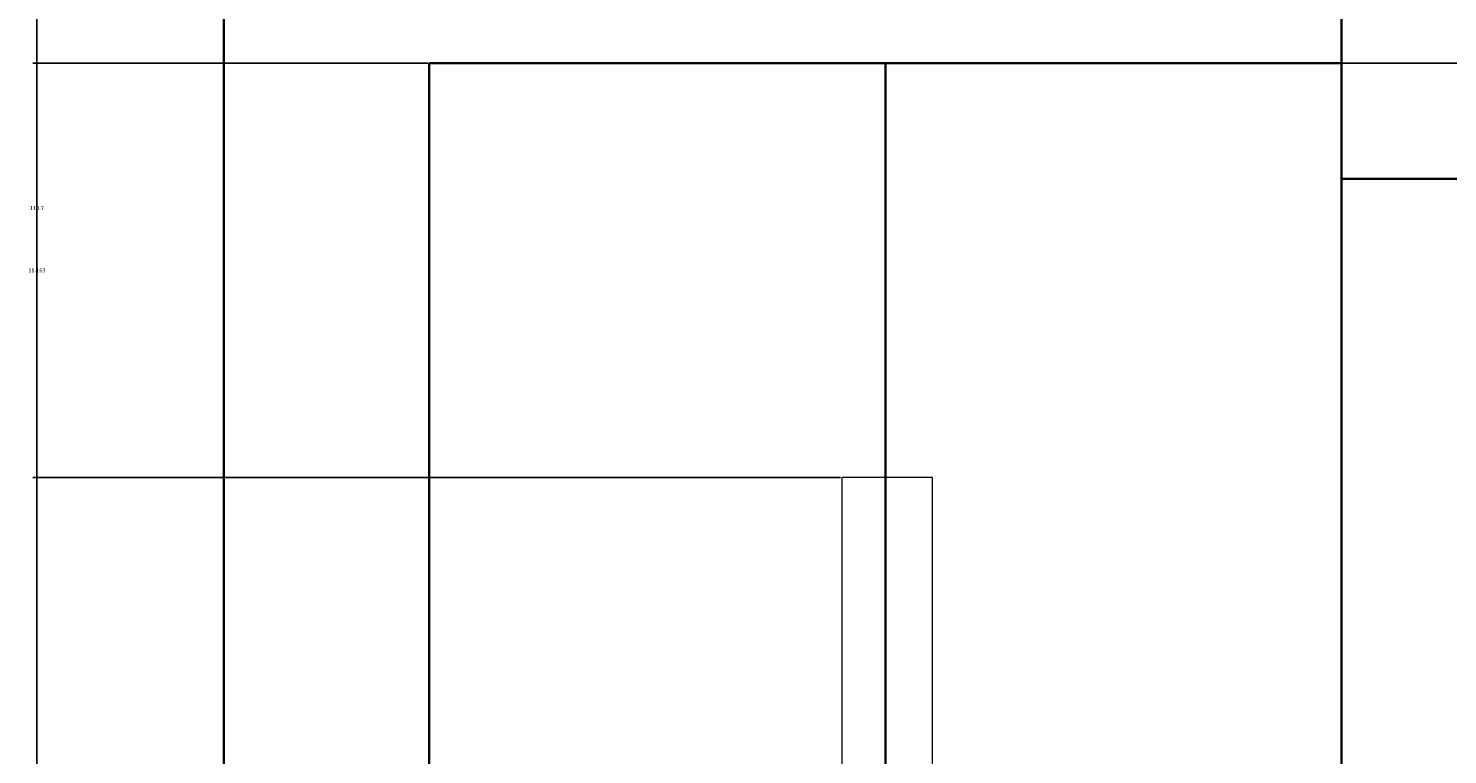
# Model space of a CAD drawing. Units: inches. Extents: x 27 to 200, y -50 to 102.
# Tile 5 of 26: x 27 to 89, y 15 to 46. Entities that reach past the tile are written whole.
import ezdxf

# ---------------------------------------------------------------- set-up
doc = ezdxf.new("R2010")
doc.units = ezdxf.units.IN
doc.header["$MEASUREMENT"] = 0
for name, color, linetype, lineweight in [('A-ANNO-DIMS', 2, 'Continuous', 18), ('A-ELEV', 7, 'Continuous', 35), ('A-EQPM', 9, 'Continuous', 18)]:
    doc.layers.add(name, color=color, linetype=linetype, lineweight=lineweight)
doc.styles.get("Standard").update_dxf_attribs({"font": 'arial.ttf'})
doc.dimstyles.get("Standard").update_dxf_attribs({"dimtxt": 0.18, "dimasz": 0.18, "dimexe": 0.18, "dimexo": 0.0625, "dimgap": 0.09, "dimtad": 0, "dimtih": 1, "dimtoh": 1, "dimdec": 4, "dimzin": 0, "dimdsep": 46, "dimtxsty": 'Standard', "dimcen": 0.09, "dimadec": 0, "dimazin": 0, "dimtfac": 1, "dimtdec": 4, "dimtofl": 0, "dimtmove": 0, "dimatfit": 3, "dimfxl": 1, "dimtolj": 1, "dimtzin": 0, "dimarcsym": 0})

# ---------------------------------------------------------------- blocks, each defined once
blk = doc.blocks.new('*D24')
at = {"layer": 'A-ANNO-DIMS', "color": 0, "lineweight": -2, "transparency": 16777216}
for p, q in [((35.354, 93.926), (27.037, 93.926)), ((27.217, 93.746), (27.217, 38.76)), ((27.217, -16.589), (27.217, 38.397)), ((35.354, -16.769), (27.037, -16.769))]:
    blk.add_line(p, q, dxfattribs=at)
at = {"layer": 'A-ANNO-DIMS', "color": 0, "transparency": 16777216}
for points in [[(27.187, 93.746), (27.247, 93.746), (27.217, 93.926)], [(27.187, -16.589), (27.247, -16.589), (27.217, -16.769)]]:
    blk.add_solid(points, dxfattribs=at)
at = {"layer": 'Defpoints', "color": 0, "transparency": 16777216}
for p in [(27.217, 93.926), (35.417, 93.926), (35.417, -16.769)]:
    blk.add_point(p, dxfattribs=at)
at = {"layer": 'A-ANNO-DIMS', "color": 0, "transparency": 16777216, "insert": (27.217, 38.579), "char_height": 0.18, "attachment_point": 5}
blk.add_mtext('\\A1;110.7', dxfattribs=at)
blk = doc.blocks.new('*D45')
at = {"layer": 'A-ANNO-DIMS', "color": 0, "lineweight": -2, "transparency": 16777216}
for p, q in [((62.443, 26.764), (27.037, 26.764)), ((27.217, 26.584), (27.217, 11.755)), ((27.217, -3.437), (27.217, 11.392)), ((62.443, -3.617), (27.037, -3.617))]:
    blk.add_line(p, q, dxfattribs=at)
at = {"layer": 'A-ANNO-DIMS', "color": 0, "transparency": 16777216}
for points in [[(27.187, 26.584), (27.247, 26.584), (27.217, 26.764)], [(27.187, -3.437), (27.247, -3.437), (27.217, -3.617)]]:
    blk.add_solid(points, dxfattribs=at)
at = {"layer": 'Defpoints', "color": 0, "transparency": 16777216}
for p in [(27.217, 26.764), (62.505, 26.764), (62.505, -3.617)]:
    blk.add_point(p, dxfattribs=at)
at = {"layer": 'A-ANNO-DIMS', "color": 0, "transparency": 16777216, "insert": (27.217, 11.573), "char_height": 0.18, "attachment_point": 5}
blk.add_mtext('\\A1;30.38', dxfattribs=at)
blk = doc.blocks.new('*D46')
at = {"layer": 'A-ANNO-DIMS', "color": 0, "lineweight": -2, "transparency": 16777216}
for p, q in [((44.354, 44.926), (27.037, 44.926)), ((27.217, 44.746), (27.217, 36.027)), ((27.217, 26.944), (27.217, 35.663)), ((62.443, 26.764), (27.037, 26.764))]:
    blk.add_line(p, q, dxfattribs=at)
at = {"layer": 'A-ANNO-DIMS', "color": 0, "transparency": 16777216}
for points in [[(27.187, 44.746), (27.247, 44.746), (27.217, 44.926)], [(27.187, 26.944), (27.247, 26.944), (27.217, 26.764)]]:
    blk.add_solid(points, dxfattribs=at)
at = {"layer": 'Defpoints', "color": 0, "transparency": 16777216}
for p in [(27.217, 44.926), (44.417, 44.926), (62.505, 26.764)]:
    blk.add_point(p, dxfattribs=at)
at = {"layer": 'A-ANNO-DIMS', "color": 0, "transparency": 16777216, "insert": (27.217, 35.845), "char_height": 0.18, "attachment_point": 5}
blk.add_mtext('\\A1;18.163', dxfattribs=at)
blk = doc.blocks.new('*D47')
at = {"layer": 'A-ANNO-DIMS', "color": 0, "lineweight": -2, "transparency": 16777216}
for p, q in [((44.354402, 51.926437), (27.036902, 51.926437)), ((27.216902, 51.746437), (27.216902, 48.606437)), ((27.216902, 45.106437), (27.216902, 48.246437)), ((44.354402, 44.926437), (27.036902, 44.926437))]:
    blk.add_line(p, q, dxfattribs=at)
at = {"layer": 'A-ANNO-DIMS', "color": 0, "transparency": 16777216}
for points in [[(27.186902, 51.746437), (27.246902, 51.746437), (27.216902, 51.926437)], [(27.186902, 45.106437), (27.246902, 45.106437), (27.216902, 44.926437)]]:
    blk.add_solid(points, dxfattribs=at)
at = {"layer": 'Defpoints', "color": 0, "transparency": 16777216}
for p in [(27.216902, 51.926437), (44.416902, 51.926437), (44.416902, 44.926437)]:
    blk.add_point(p, dxfattribs=at)
at = {"layer": 'A-ANNO-DIMS', "color": 0, "transparency": 16777216, "insert": (27.216902, 48.426437), "char_height": 0.18, "attachment_point": 5}
blk.add_mtext('\\A1;7', dxfattribs=at)
blk = doc.blocks.new('*D48')
at = {"layer": 'A-ANNO-DIMS', "color": 0, "lineweight": -2, "transparency": 16777216}
for p, q in [((84.479, 44.926), (199.797, 44.926)), ((199.617, 44.746), (199.617, 14.26)), ((199.617, -16.589), (199.617, 13.897)), ((84.479, -16.769), (199.797, -16.769))]:
    blk.add_line(p, q, dxfattribs=at)
at = {"layer": 'A-ANNO-DIMS', "color": 0, "transparency": 16777216}
for points in [[(199.587, 44.746), (199.647, 44.746), (199.617, 44.926)], [(199.587, -16.589), (199.647, -16.589), (199.617, -16.769)]]:
    blk.add_solid(points, dxfattribs=at)
at = {"layer": 'Defpoints', "color": 0, "transparency": 16777216}
for p in [(84.417, 44.926), (199.617, 44.926), (84.417, -16.769)]:
    blk.add_point(p, dxfattribs=at)
at = {"layer": 'A-ANNO-DIMS', "color": 0, "transparency": 16777216, "insert": (199.617, 14.079), "char_height": 0.18, "attachment_point": 5}
blk.add_mtext('\\A1;61.7', dxfattribs=at)

msp = doc.modelspace()

# ---------------------------------------------------------------- linework, layer by layer
at = {"layer": 'A-ELEV'}
for p, q in [((35.4169, 93.9264), (35.4169, -16.7693)), ((44.4169, 44.9264), (44.4169, -16.7693)), ((84.4169, 44.9264), (44.4169, 44.9264)), ((64.4169, 44.9264), (64.4169, -16.7693)), ((84.4169, 44.9264), (84.4169, -16.7693))]:
    msp.add_line(p, q, dxfattribs=at)
msp.add_lwpolyline([(84.4169, 65.5865), (120.4169, 65.5865), (120.4169, 39.8559), (84.4169, 39.8559)], close=True, dxfattribs=at)
at = {"layer": 'A-EQPM'}
for points in [[(64.4169, 26.7638), (62.5054, 26.7638), (62.5054, -3.6168), (64.4169, -3.6168)], [(64.4169, -3.6168), (66.4786, -3.6168), (66.4786, 26.7638), (64.4169, 26.7638)]]:
    msp.add_lwpolyline(points, close=True, dxfattribs=at)

# ---------------------------------------------------------------- dimensions: what is measured, and where the dimension line sits
at = {"layer": 'A-ANNO-DIMS'}
for base, p1, p2, override, picture, middle in [((27.2169, 93.9264), (35.4169, -16.7693), (35.4169, 93.9264), {"dimdec": 1, "dimlfac": 1, "dimrnd": 0, "dimzin": 0, "dimdsep": 46, "dimlunit": 2}, '*D24', (27.2169, 38.5786)), ((27.2169, 51.9264), (44.4169, 44.9264), (44.4169, 51.9264), {"dimdec": 0, "dimlfac": 1, "dimrnd": 0, "dimzin": 0, "dimdsep": 46, "dimlunit": 2}, '*D47', (27.2169, 48.4264)), ((27.2169, 44.9264), (62.5054, 26.7638), (44.4169, 44.9264), {"dimdec": 3, "dimlfac": 1, "dimrnd": 0, "dimzin": 0, "dimdsep": 46, "dimlunit": 2}, '*D46', (27.2169, 35.8451)), ((199.6169, 44.9264), (84.4169, -16.7693), (84.4169, 44.9264), {"dimdec": 1, "dimlfac": 1, "dimrnd": 0, "dimzin": 0, "dimdsep": 46, "dimlunit": 2}, '*D48', (199.6169, 14.0786)), ((27.2169, 26.7638), (62.5054, -3.6168), (62.5054, 26.7638), {"dimdec": 2, "dimlfac": 1, "dimrnd": 0, "dimzin": 0, "dimdsep": 46, "dimlunit": 2}, '*D45', (27.2169, 11.5735))]:
    dim = msp.add_linear_dim(base=base, p1=p1, p2=p2, angle=90, dimstyle='Standard', override=override, dxfattribs=at)
    dim.commit()
    dim.dimension.update_dxf_attribs({"geometry": picture, "text_midpoint": middle})

doc.saveas('drawing.dxf')
